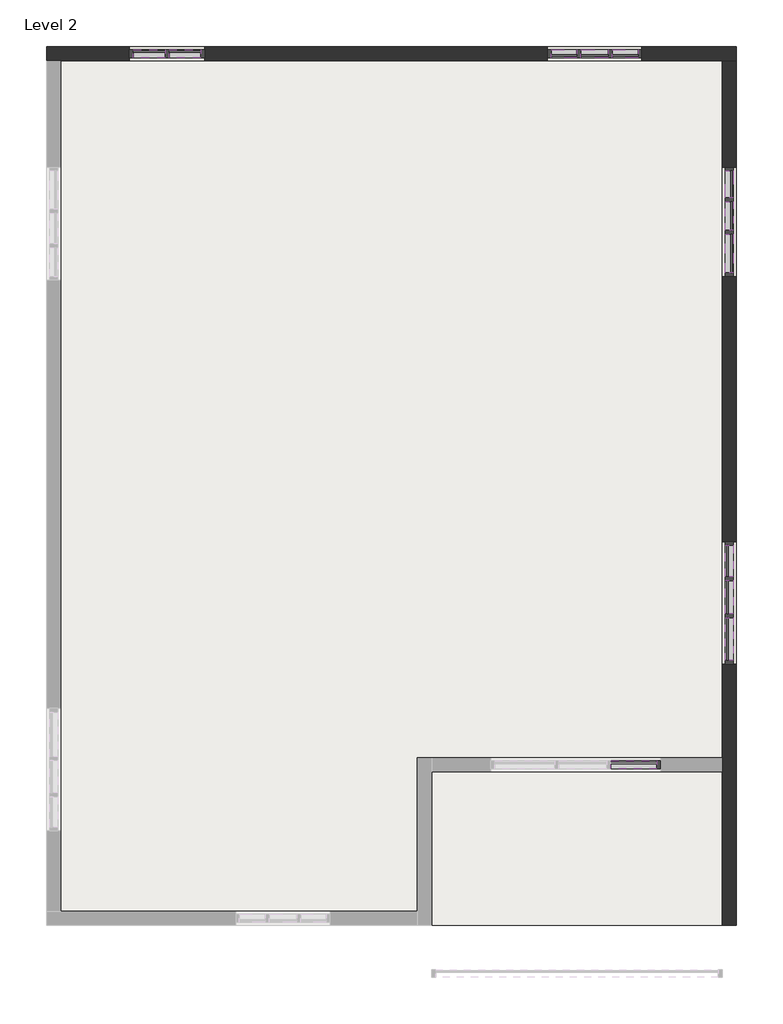
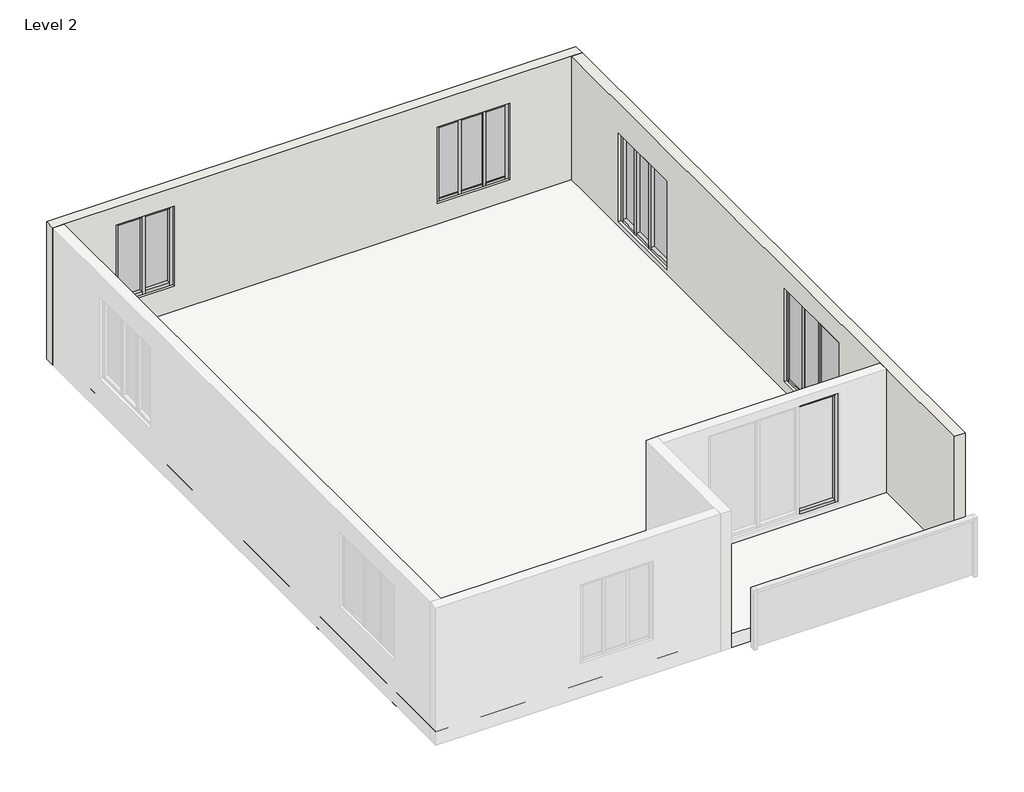
# One storey, part 2 of 2: 40 members, 11 plates, 2 walls, 1 roof.
"""IFC4 building model written with IfcOpenShell, lengths in millimetres."""

from ifc_helpers import new_model, si_unit, frame, origin, place, context, project, spatial, polyline, outline, extrude, faceted_brep, transform, mapped, element, save
from components import member_dc106669, member_0b7646a3, member_5f1d7e17, member_3f0e0172, member_3a0a7659, member_e878716d, member_b281fab0, member_45f9c1ec, member_8ea2817a, member_8eaddbd8, member_5535eeb3, member_69a911c1, member_1f3b6741, member_0bd10330, member_bc7dbe04, member_cf2a6f2c, member_fe0bf6b7, member_58f5e783, member_c04b3d4e, system_panel_glazed_4740d582, system_panel_glazed_d76279c0, system_panel_glazed_83f38206, system_panel_glazed_f7c25410, system_panel_glazed_1587745b, system_panel_glazed_2a40583e, system_panel_glazed_9aad7cd6, system_panel_glazed_e232d9b5, system_panel_glazed_0947b60d

model = new_model("IFC4")

# Units and contexts
model_context = context("Model", 3, world=origin())
ifc_project = project(units=[si_unit("LENGTHUNIT", "METRE", prefix="MILLI")], contexts=[model_context])

# Site, building, storey
site = spatial("IfcSite", under=ifc_project)
building = spatial("IfcBuilding", under=site)
storey = spatial("IfcBuildingStorey", under=building, Name="Level 2", Elevation=3048.0)

# Members
placement = place(None, origin())
member_shape = member_dc106669(model_context)
element("IfcMember", 1, ObjectType="Rectangular Mullion : 2.5\" x 5\" rectangular", at=placement, inside=storey, context=model_context, shape_type="MappedRepresentation", body=[
    mapped(member_shape, transform((-7605.3781629, -790.0678064, 5503.2729534), x_axis=(0.0, 0.0, 1.0), y_axis=(0.0, 1.0, 0.0), z_axis=(-1.0, 0.0, 0.0))),
])
element("IfcMember", 2, ObjectType="Rectangular Mullion : 2.5\" x 5\" rectangular", at=placement, inside=storey, context=model_context, shape_type="MappedRepresentation", body=[
    mapped(member_shape, transform((-8589.6281629, -790.0678064, 5503.2729534), x_axis=(0.0, 0.0, 1.0), y_axis=(0.0, 1.0, 0.0), z_axis=(-1.0, 0.0, 0.0))),
])
element("IfcMember", 3, ObjectType="Rectangular Mullion : 2.5\" x 5\" rectangular", at=placement, inside=storey, context=model_context, shape_type="MappedRepresentation", body=[
    mapped(member_shape, transform((-8176.8781629, -790.0678064, 3807.0200841), x_axis=(0.0, 0.0, -1.0), y_axis=(0.0, 1.0, 0.0), z_axis=(1.0, 0.0, 0.0))),
])
element("IfcMember", 4, ObjectType="Rectangular Mullion : 2.5\" x 5\" rectangular", at=placement, inside=storey, context=model_context, shape_type="MappedRepresentation", body=[
    mapped(member_shape, transform((-7192.6281629, -790.0678064, 3807.0200841), x_axis=(0.0, 0.0, -1.0), y_axis=(0.0, 1.0, 0.0), z_axis=(1.0, 0.0, 0.0))),
])
member_2_shape = member_0b7646a3(model_context)
element("IfcMember", 5, ObjectType="Rectangular Mullion : 2.5\" x 5\" rectangular", at=placement, inside=storey, context=model_context, shape_type="MappedRepresentation", body=[
    mapped(member_2_shape, transform((-14818.9781629, -790.0678064, 5692.341576), x_axis=(0.0, 0.0, 1.0), y_axis=(0.0, -1.0, 0.0), z_axis=(1.0, 0.0, 0.0))),
])
element("IfcMember", 6, ObjectType="Rectangular Mullion : 2.5\" x 5\" rectangular", at=placement, inside=storey, context=model_context, shape_type="MappedRepresentation", body=[
    mapped(member_2_shape, transform((-14241.1281629, -790.0678064, 5692.341576), x_axis=(0.0, 0.0, 1.0), y_axis=(0.0, -1.0, 0.0), z_axis=(1.0, 0.0, 0.0))),
])
element("IfcMember", 7, ObjectType="Rectangular Mullion : 2.5\" x 5\" rectangular", at=placement, inside=storey, context=model_context, shape_type="MappedRepresentation", body=[
    mapped(member_2_shape, transform((-14755.4781629, -790.0678064, 3913.1194519), x_axis=(0.0, 0.0, -1.0), y_axis=(0.0, -1.0, 0.0), z_axis=(-1.0, 0.0, 0.0))),
])
element("IfcMember", 8, ObjectType="Rectangular Mullion : 2.5\" x 5\" rectangular", at=placement, inside=storey, context=model_context, shape_type="MappedRepresentation", body=[
    mapped(member_2_shape, transform((-15333.3281629, -790.0678064, 3913.1194519), x_axis=(0.0, 0.0, -1.0), y_axis=(0.0, -1.0, 0.0), z_axis=(-1.0, 0.0, 0.0))),
])
member_3_shape = member_5f1d7e17(model_context)
element("IfcMember", 9, ObjectType="Rectangular Mullion : 2.5\" x 5\" rectangular", at=placement, inside=storey, context=model_context, shape_type="MappedRepresentation", body=[
    mapped(member_3_shape, transform((-5719.4281629, -9883.2678064, 5635.9695852), x_axis=(0.0, 0.0, 1.0), y_axis=(1.0, 0.0, 0.0), z_axis=(0.0, 1.0, 0.0))),
])
element("IfcMember", 10, ObjectType="Rectangular Mullion : 2.5\" x 5\" rectangular", at=placement, inside=storey, context=model_context, shape_type="MappedRepresentation", body=[
    mapped(member_3_shape, transform((-5719.4281629, -10575.4178064, 3572.3548103), x_axis=(0.0, 0.0, -1.0), y_axis=(1.0, 0.0, 0.0), z_axis=(0.0, -1.0, 0.0))),
])
member_4_shape = member_3f0e0172(model_context)
element("IfcMember", 11, ObjectType="Rectangular Mullion : 2.5\" x 5\" rectangular", at=placement, inside=storey, context=model_context, shape_type="MappedRepresentation", body=[
    mapped(member_4_shape, transform((-5719.4281629, -3704.7178064, 3463.7409857), x_axis=(0.0, 0.0, -1.0), y_axis=(-1.0, 0.0, 0.0), z_axis=(0.0, 1.0, 0.0))),
])
member_5_shape = member_3a0a7659(model_context)
element("IfcMember", 12, ObjectType="Rectangular Mullion : 2.5\" x 5\" rectangular", at=placement, inside=storey, context=model_context, shape_type="MappedRepresentation", body=[
    mapped(member_5_shape, transform((-7630.7781629, -12258.1678064, 3466.2078322), x_axis=(0.0, 0.0, -1.0), y_axis=(0.0, -1.0, 0.0), z_axis=(-1.0, 0.0, 0.0))),
])
element("IfcMember", 13, ObjectType="Rectangular Mullion : 2.5\" x 5\" rectangular", at=placement, inside=storey, context=model_context, shape_type="MappedRepresentation", body=[
    mapped(member_5_shape, transform((-6887.8281629, -12258.1678064, 5911.9599258), x_axis=(0.0, 0.0, 1.0), y_axis=(0.0, -1.0, 0.0), z_axis=(1.0, 0.0, 0.0))),
])
element("IfcMember", 14, ObjectType="Rectangular Mullion : 2.5\" x 5\" rectangular", at=placement, inside=storey, context=model_context, shape_type="MappedRepresentation", body=[
    mapped(member_4_shape, transform((-5719.4281629, -4320.6678064, 5428.2301601), x_axis=(0.0, 0.0, 1.0), y_axis=(-1.0, 0.0, 0.0), z_axis=(0.0, -1.0, 0.0))),
])
member_6_shape = member_e878716d(model_context)
element("IfcMember", 15, ObjectType="Rectangular Mullion : 2.5\" x 5\" rectangular", at=placement, inside=storey, context=model_context, shape_type="MappedRepresentation", body=[
    mapped(member_6_shape, transform((-6824.3281629, -12258.1678064, 3466.2078322), x_axis=(1.0, 0.0, 0.0), y_axis=(0.0, -1.0, 0.0), z_axis=(0.0, 0.0, -1.0))),
])
member_7_shape = member_b281fab0(model_context)
element("IfcMember", 16, ObjectType="Rectangular Mullion : 2.5\" x 5\" rectangular", at=placement, inside=storey, context=model_context, shape_type="MappedRepresentation", body=[
    mapped(member_7_shape, transform((-5719.4281629, -9286.3678064, 5635.9695852), x_axis=(0.0, 0.0, 1.0), y_axis=(1.0, 0.0, 0.0), z_axis=(0.0, 1.0, 0.0))),
])
member_8_shape = member_45f9c1ec(model_context)
element("IfcMember", 17, ObjectType="Rectangular Mullion : 2.5\" x 5\" rectangular", at=placement, inside=storey, context=model_context, shape_type="MappedRepresentation", body=[
    mapped(member_8_shape, transform((-5719.4281629, -8721.2178064, 5635.9695852), x_axis=(0.0, 0.0, 1.0), y_axis=(1.0, 0.0, 0.0), z_axis=(0.0, 1.0, 0.0))),
])
member_9_shape = member_8ea2817a(model_context)
element("IfcMember", 18, ObjectType="Rectangular Mullion : 2.5\" x 5\" rectangular", at=placement, inside=storey, context=model_context, shape_type="MappedRepresentation", body=[
    mapped(member_9_shape, transform((-5719.4281629, -9254.6178064, 3572.3548103), x_axis=(0.0, 1.0, 0.0), y_axis=(1.0, 0.0, 0.0), z_axis=(0.0, 0.0, -1.0))),
])
element("IfcMember", 19, ObjectType="Rectangular Mullion : 2.5\" x 5\" rectangular", at=placement, inside=storey, context=model_context, shape_type="MappedRepresentation", body=[
    mapped(member_9_shape, transform((-5719.4281629, -9851.5178064, 3572.3548103), x_axis=(0.0, 1.0, 0.0), y_axis=(1.0, 0.0, 0.0), z_axis=(0.0, 0.0, -1.0))),
])
element("IfcMember", 20, ObjectType="Rectangular Mullion : 2.5\" x 5\" rectangular", at=placement, inside=storey, context=model_context, shape_type="MappedRepresentation", body=[
    mapped(member_8_shape, transform((-5719.4281629, -9222.8678064, 3572.3548103), x_axis=(0.0, 0.0, -1.0), y_axis=(1.0, 0.0, 0.0), z_axis=(0.0, -1.0, 0.0))),
])
element("IfcMember", 21, ObjectType="Rectangular Mullion : 2.5\" x 5\" rectangular", at=placement, inside=storey, context=model_context, shape_type="MappedRepresentation", body=[
    mapped(member_7_shape, transform((-5719.4281629, -9819.7678064, 3572.3548103), x_axis=(0.0, 0.0, -1.0), y_axis=(1.0, 0.0, 0.0), z_axis=(0.0, -1.0, 0.0))),
])
member_10_shape = member_8eaddbd8(model_context)
element("IfcMember", 22, ObjectType="Rectangular Mullion : 2.5\" x 5\" rectangular", at=placement, inside=storey, context=model_context, shape_type="MappedRepresentation", body=[
    mapped(member_10_shape, transform((-5719.4281629, -8657.7178064, 3572.3548103), x_axis=(0.0, 1.0, 0.0), y_axis=(1.0, 0.0, 0.0), z_axis=(0.0, 0.0, -1.0))),
])
element("IfcMember", 23, ObjectType="Rectangular Mullion : 2.5\" x 5\" rectangular", at=placement, inside=storey, context=model_context, shape_type="MappedRepresentation", body=[
    mapped(member_10_shape, transform((-5719.4281629, -10638.9178064, 5635.9695852), x_axis=(0.0, -1.0, 0.0), y_axis=(1.0, 0.0, 0.0), z_axis=(0.0, 0.0, 1.0))),
])
member_11_shape = member_5535eeb3(model_context)
element("IfcMember", 24, ObjectType="Rectangular Mullion : 2.5\" x 5\" rectangular", at=placement, inside=storey, context=model_context, shape_type="MappedRepresentation", body=[
    mapped(member_11_shape, transform((-5719.4281629, -3177.6678064, 3463.7409857), x_axis=(0.0, 0.0, -1.0), y_axis=(-1.0, 0.0, 0.0), z_axis=(0.0, 1.0, 0.0))),
])
member_12_shape = member_69a911c1(model_context)
element("IfcMember", 25, ObjectType="Rectangular Mullion : 2.5\" x 5\" rectangular", at=placement, inside=storey, context=model_context, shape_type="MappedRepresentation", body=[
    mapped(member_12_shape, transform((-5719.4281629, -2682.3678064, 3463.7409857), x_axis=(0.0, 0.0, -1.0), y_axis=(-1.0, 0.0, 0.0), z_axis=(0.0, 1.0, 0.0))),
])
member_13_shape = member_1f3b6741(model_context)
element("IfcMember", 26, ObjectType="Rectangular Mullion : 2.5\" x 5\" rectangular", at=placement, inside=storey, context=model_context, shape_type="MappedRepresentation", body=[
    mapped(member_13_shape, transform((-5719.4281629, -3145.9178064, 3463.7409857), x_axis=(0.0, -1.0, 0.0), y_axis=(-1.0, 0.0, 0.0), z_axis=(0.0, 0.0, -1.0))),
])
element("IfcMember", 27, ObjectType="Rectangular Mullion : 2.5\" x 5\" rectangular", at=placement, inside=storey, context=model_context, shape_type="MappedRepresentation", body=[
    mapped(member_13_shape, transform((-5719.4281629, -3672.9678064, 3463.7409857), x_axis=(0.0, -1.0, 0.0), y_axis=(-1.0, 0.0, 0.0), z_axis=(0.0, 0.0, -1.0))),
])
element("IfcMember", 28, ObjectType="Rectangular Mullion : 2.5\" x 5\" rectangular", at=placement, inside=storey, context=model_context, shape_type="MappedRepresentation", body=[
    mapped(member_12_shape, transform((-5719.4281629, -3114.1678064, 5428.2301601), x_axis=(0.0, 0.0, 1.0), y_axis=(-1.0, 0.0, 0.0), z_axis=(0.0, -1.0, 0.0))),
])
element("IfcMember", 29, ObjectType="Rectangular Mullion : 2.5\" x 5\" rectangular", at=placement, inside=storey, context=model_context, shape_type="MappedRepresentation", body=[
    mapped(member_11_shape, transform((-5719.4281629, -3641.2178064, 5428.2301601), x_axis=(0.0, 0.0, 1.0), y_axis=(-1.0, 0.0, 0.0), z_axis=(0.0, -1.0, 0.0))),
])
member_14_shape = member_0bd10330(model_context)
element("IfcMember", 30, ObjectType="Rectangular Mullion : 2.5\" x 5\" rectangular", at=placement, inside=storey, context=model_context, shape_type="MappedRepresentation", body=[
    mapped(member_14_shape, transform((-5719.4281629, -2618.8678064, 5428.2301601), x_axis=(0.0, 1.0, 0.0), y_axis=(-1.0, 0.0, 0.0), z_axis=(0.0, 0.0, 1.0))),
])
element("IfcMember", 31, ObjectType="Rectangular Mullion : 2.5\" x 5\" rectangular", at=placement, inside=storey, context=model_context, shape_type="MappedRepresentation", body=[
    mapped(member_14_shape, transform((-5719.4281629, -4384.1678064, 3463.7409857), x_axis=(0.0, -1.0, 0.0), y_axis=(-1.0, 0.0, 0.0), z_axis=(0.0, 0.0, -1.0))),
])
member_15_shape = member_bc7dbe04(model_context)
element("IfcMember", 32, ObjectType="Rectangular Mullion : 2.5\" x 5\" rectangular", at=placement, inside=storey, context=model_context, shape_type="MappedRepresentation", body=[
    mapped(member_15_shape, transform((-7668.8781629, -790.0678064, 3807.0200841), x_axis=(0.0, 0.0, -1.0), y_axis=(0.0, 1.0, 0.0), z_axis=(1.0, 0.0, 0.0))),
])
member_16_shape = member_cf2a6f2c(model_context)
element("IfcMember", 33, ObjectType="Rectangular Mullion : 2.5\" x 5\" rectangular", at=placement, inside=storey, context=model_context, shape_type="MappedRepresentation", body=[
    mapped(member_16_shape, transform((-7637.1281629, -790.0678064, 3807.0200841), x_axis=(-1.0, 0.0, 0.0), y_axis=(0.0, 1.0, 0.0), z_axis=(0.0, 0.0, -1.0))),
])
element("IfcMember", 34, ObjectType="Rectangular Mullion : 2.5\" x 5\" rectangular", at=placement, inside=storey, context=model_context, shape_type="MappedRepresentation", body=[
    mapped(member_16_shape, transform((-8145.1281629, -790.0678064, 3807.0200841), x_axis=(-1.0, 0.0, 0.0), y_axis=(0.0, 1.0, 0.0), z_axis=(0.0, 0.0, -1.0))),
])
element("IfcMember", 35, ObjectType="Rectangular Mullion : 2.5\" x 5\" rectangular", at=placement, inside=storey, context=model_context, shape_type="MappedRepresentation", body=[
    mapped(member_15_shape, transform((-8113.3781629, -790.0678064, 5503.2729534), x_axis=(0.0, 0.0, 1.0), y_axis=(0.0, 1.0, 0.0), z_axis=(-1.0, 0.0, 0.0))),
])
member_17_shape = member_fe0bf6b7(model_context)
element("IfcMember", 36, ObjectType="Rectangular Mullion : 2.5\" x 5\" rectangular", at=placement, inside=storey, context=model_context, shape_type="MappedRepresentation", body=[
    mapped(member_17_shape, transform((-8653.1281629, -790.0678064, 3807.0200841), x_axis=(-1.0, 0.0, 0.0), y_axis=(0.0, 1.0, 0.0), z_axis=(0.0, 0.0, -1.0))),
])
element("IfcMember", 37, ObjectType="Rectangular Mullion : 2.5\" x 5\" rectangular", at=placement, inside=storey, context=model_context, shape_type="MappedRepresentation", body=[
    mapped(member_17_shape, transform((-7129.1281629, -790.0678064, 5503.2729534), x_axis=(1.0, 0.0, 0.0), y_axis=(0.0, 1.0, 0.0), z_axis=(0.0, 0.0, 1.0))),
])
member_18_shape = member_58f5e783(model_context)
element("IfcMember", 38, ObjectType="Rectangular Mullion : 2.5\" x 5\" rectangular", at=placement, inside=storey, context=model_context, shape_type="MappedRepresentation", body=[
    mapped(member_18_shape, transform((-14787.2281629, -790.0678064, 3913.1194519), x_axis=(1.0, 0.0, 0.0), y_axis=(0.0, -1.0, 0.0), z_axis=(0.0, 0.0, -1.0))),
])
member_19_shape = member_c04b3d4e(model_context)
element("IfcMember", 39, ObjectType="Rectangular Mullion : 2.5\" x 5\" rectangular", at=placement, inside=storey, context=model_context, shape_type="MappedRepresentation", body=[
    mapped(member_19_shape, transform((-15396.8281629, -790.0678064, 5692.341576), x_axis=(-1.0, 0.0, 0.0), y_axis=(0.0, -1.0, 0.0), z_axis=(0.0, 0.0, 1.0))),
])
element("IfcMember", 40, ObjectType="Rectangular Mullion : 2.5\" x 5\" rectangular", at=placement, inside=storey, context=model_context, shape_type="MappedRepresentation", body=[
    mapped(member_19_shape, transform((-14177.6281629, -790.0678064, 3913.1194519), x_axis=(1.0, 0.0, 0.0), y_axis=(0.0, -1.0, 0.0), z_axis=(0.0, 0.0, -1.0))),
])

# Plates
system_panel_glazed_shape = system_panel_glazed_4740d582(model_context)
element("IfcPlate", 41, ObjectType="System Panel : Glazed", at=placement, inside=storey, context=model_context, shape_type="MappedRepresentation", body=[
    mapped(system_panel_glazed_shape, transform((-5719.4281629, -10229.3428064, 3635.8548103), x_axis=(0.0, 1.0, 0.0), y_axis=(-1.0, 0.0, 0.0), z_axis=(0.0, 0.0, 1.0))),
])
system_panel_glazed_2_shape = system_panel_glazed_d76279c0(model_context)
element("IfcPlate", 42, ObjectType="System Panel : Glazed", at=placement, inside=storey, context=model_context, shape_type="MappedRepresentation", body=[
    mapped(system_panel_glazed_2_shape, transform((-5719.4281629, -9553.0678064, 3635.8548103), x_axis=(0.0, 1.0, 0.0), y_axis=(-1.0, 0.0, 0.0), z_axis=(0.0, 0.0, 1.0))),
])
system_panel_glazed_3_shape = system_panel_glazed_83f38206(model_context)
element("IfcPlate", 43, ObjectType="System Panel : Glazed", at=placement, inside=storey, context=model_context, shape_type="MappedRepresentation", body=[
    mapped(system_panel_glazed_3_shape, transform((-5719.4281629, -8972.0428064, 3635.8548103), x_axis=(0.0, 1.0, 0.0), y_axis=(-1.0, 0.0, 0.0), z_axis=(0.0, 0.0, 1.0))),
])
system_panel_glazed_4_shape = system_panel_glazed_f7c25410(model_context)
element("IfcPlate", 44, ObjectType="System Panel : Glazed", at=placement, inside=storey, context=model_context, shape_type="MappedRepresentation", body=[
    mapped(system_panel_glazed_4_shape, transform((-5719.4281629, -2898.2678064, 3527.2409857), x_axis=(0.0, -1.0, 0.0), y_axis=(1.0, 0.0, 0.0), z_axis=(0.0, 0.0, 1.0))),
])
system_panel_glazed_5_shape = system_panel_glazed_1587745b(model_context)
element("IfcPlate", 45, ObjectType="System Panel : Glazed", at=placement, inside=storey, context=model_context, shape_type="MappedRepresentation", body=[
    mapped(system_panel_glazed_5_shape, transform((-5719.4281629, -4012.6928064, 3527.2409857), x_axis=(0.0, -1.0, 0.0), y_axis=(1.0, 0.0, 0.0), z_axis=(0.0, 0.0, 1.0))),
])
system_panel_glazed_6_shape = system_panel_glazed_2a40583e(model_context)
element("IfcPlate", 46, ObjectType="System Panel : Glazed", at=placement, inside=storey, context=model_context, shape_type="MappedRepresentation", body=[
    mapped(system_panel_glazed_6_shape, transform((-5719.4281629, -3409.4428064, 3527.2409857), x_axis=(0.0, -1.0, 0.0), y_axis=(1.0, 0.0, 0.0), z_axis=(0.0, 0.0, 1.0))),
])
system_panel_glazed_7_shape = system_panel_glazed_9aad7cd6(model_context)
element("IfcPlate", 47, ObjectType="System Panel : Glazed", at=placement, inside=storey, context=model_context, shape_type="MappedRepresentation", body=[
    mapped(system_panel_glazed_7_shape, transform((-7399.0031629, -790.0678064, 3870.5200841), x_axis=(-1.0, 0.0, 0.0), y_axis=(0.0, -1.0, 0.0), z_axis=(0.0, 0.0, 1.0))),
])
element("IfcPlate", 48, ObjectType="System Panel : Glazed", at=placement, inside=storey, context=model_context, shape_type="MappedRepresentation", body=[
    mapped(system_panel_glazed_7_shape, transform((-8383.2531629, -790.0678064, 3870.5200841), x_axis=(-1.0, 0.0, 0.0), y_axis=(0.0, -1.0, 0.0), z_axis=(0.0, 0.0, 1.0))),
])
system_panel_glazed_8_shape = system_panel_glazed_e232d9b5(model_context)
element("IfcPlate", 49, ObjectType="System Panel : Glazed", at=placement, inside=storey, context=model_context, shape_type="MappedRepresentation", body=[
    mapped(system_panel_glazed_8_shape, transform((-7891.1281629, -790.0678064, 3870.5200841), x_axis=(-1.0, 0.0, 0.0), y_axis=(0.0, -1.0, 0.0), z_axis=(0.0, 0.0, 1.0))),
])
system_panel_glazed_9_shape = system_panel_glazed_0947b60d(model_context)
element("IfcPlate", 50, ObjectType="System Panel : Glazed", at=placement, inside=storey, context=model_context, shape_type="MappedRepresentation", body=[
    mapped(system_panel_glazed_9_shape, transform((-15076.1531629, -790.0678064, 3976.6194519), x_axis=(1.0, 0.0, 0.0), y_axis=(0.0, 1.0, 0.0), z_axis=(0.0, 0.0, 1.0))),
])
element("IfcPlate", 51, ObjectType="System Panel : Glazed", at=placement, inside=storey, context=model_context, shape_type="MappedRepresentation", body=[
    mapped(system_panel_glazed_9_shape, transform((-14498.3031629, -790.0678064, 3976.6194519), x_axis=(1.0, 0.0, 0.0), y_axis=(0.0, 1.0, 0.0), z_axis=(0.0, 0.0, 1.0))),
])

# Roof
element("IfcRoof", 52, ObjectType="Generic - 12\"", at=placement, inside=storey, context=model_context, shape_type="SweptSolid", body=[
    extrude(outline(polyline([(-16730.3281629, -675.7678064), (-5605.1281629, -675.7678064), (-5605.1281629, -14848.9678064), (-16730.3281629, -14848.9678064), (-16730.3281629, -675.7678064)])), frame((0.0, 0.0, 3048.0), z_axis=(0.0, 0.0, 1.0), x_axis=(1.0, 0.0, 0.0)), (0.0, 0.0, 1.0), 304.8),
])

# Walls
element("IfcWall", 53, ObjectType="9\"", at=placement, inside=storey, context=model_context, shape_type="Brep", body=[
    faceted_brep([(-16730.3281629, -904.3678064, 3048.0), (-16501.7281629, -904.3678064, 3048.0), (-5833.7281629, -904.3678064, 3048.0), (-5605.1281629, -904.3678064, 3048.0), (-5605.1281629, -904.3678064, 6096.0), (-5833.7281629, -904.3678064, 6096.0), (-16501.7281629, -904.3678064, 6096.0), (-16730.3281629, -904.3678064, 6096.0), (-7129.1281629, -904.3678064, 5503.2729534), (-7129.1281629, -904.3678064, 3807.0200841), (-8653.1281629, -904.3678064, 3807.0200841), (-8653.1281629, -904.3678064, 5503.2729534), (-15396.8281629, -904.3678064, 3913.1194519), (-15396.8281629, -904.3678064, 5692.341576), (-14177.6281629, -904.3678064, 5692.341576), (-14177.6281629, -904.3678064, 3913.1194519), (-5605.1281629, -675.7678064, 3048.0), (-16730.3281629, -675.7678064, 3048.0), (-16730.3281629, -675.7678064, 6096.0), (-5605.1281629, -675.7678064, 6096.0), (-7129.1281629, -675.7678064, 3807.0200841), (-7129.1281629, -675.7678064, 5503.2729534), (-8653.1281629, -675.7678064, 5503.2729534), (-8653.1281629, -675.7678064, 3807.0200841), (-15396.8281629, -675.7678064, 5692.341576), (-15396.8281629, -675.7678064, 3913.1194519), (-14177.6281629, -675.7678064, 3913.1194519), (-14177.6281629, -675.7678064, 5692.341576)], [[[0, 1, 2, 3, 4, 5, 6, 7], [8, 9, 10, 11], [12, 13, 14, 15]], [[16, 17, 18, 19], [20, 21, 22, 23], [24, 25, 26, 27]], [[3, 2, 1, 0, 17, 16]], [[7, 6, 5, 4, 19, 18]], [[0, 7, 18, 17]], [[4, 3, 16, 19]], [[8, 21, 20, 9]], [[21, 8, 11, 22]], [[22, 11, 10, 23]], [[9, 20, 23, 10]], [[12, 25, 24, 13]], [[13, 24, 27, 14]], [[14, 27, 26, 15]], [[25, 12, 15, 26]]]),
])
element("IfcWall", 54, ObjectType="9\"", at=placement, inside=storey, context=model_context, shape_type="Brep", body=[
    faceted_brep([(-5833.7281629, -904.3678064, 3048.0), (-5833.7281629, -12143.8678064, 3048.0), (-5833.7281629, -12372.4678064, 3048.0), (-5833.7281629, -14848.9678064, 3048.0), (-5833.7281629, -14848.9678064, 6096.0), (-5833.7281629, -12372.4678064, 6096.0), (-5833.7281629, -12143.8678064, 6096.0), (-5833.7281629, -904.3678064, 6096.0), (-5833.7281629, -10638.9178064, 5635.9695852), (-5833.7281629, -10638.9178064, 3572.3548103), (-5833.7281629, -8657.7178064, 3572.3548103), (-5833.7281629, -8657.7178064, 5635.9695852), (-5833.7281629, -2618.8678064, 3463.7409857), (-5833.7281629, -2618.8678064, 5428.2301601), (-5833.7281629, -4384.1678064, 5428.2301601), (-5833.7281629, -4384.1678064, 3463.7409857), (-5605.1281629, -14848.9678064, 3048.0), (-5605.1281629, -904.3678064, 3048.0), (-5605.1281629, -904.3678064, 6096.0), (-5605.1281629, -14848.9678064, 6096.0), (-5605.1281629, -10638.9178064, 3572.3548103), (-5605.1281629, -10638.9178064, 5635.9695852), (-5605.1281629, -8657.7178064, 5635.9695852), (-5605.1281629, -8657.7178064, 3572.3548103), (-5605.1281629, -2618.8678064, 5428.2301601), (-5605.1281629, -2618.8678064, 3463.7409857), (-5605.1281629, -4384.1678064, 3463.7409857), (-5605.1281629, -4384.1678064, 5428.2301601)], [[[0, 1, 2, 3, 4, 5, 6, 7], [8, 9, 10, 11], [12, 13, 14, 15]], [[16, 17, 18, 19], [20, 21, 22, 23], [24, 25, 26, 27]], [[3, 2, 1, 0, 17, 16]], [[4, 3, 16, 19]], [[7, 6, 5, 4, 19, 18]], [[0, 7, 18, 17]], [[8, 21, 20, 9]], [[21, 8, 11, 22]], [[22, 11, 10, 23]], [[9, 20, 23, 10]], [[12, 25, 24, 13]], [[13, 24, 27, 14]], [[14, 27, 26, 15]], [[25, 12, 15, 26]]]),
])

save(model, "model.ifc")

# Revit data of these elements
# Type "Rectangular Mullion : 2.5\" x 5\" rectangular"
#   built-in parameter 1007304 = 0.416667 (stored number, unit not read)
#   built-in parameter 1007301 = 0.104167 (stored number, unit not read)
#   built-in parameter 1007300 = 0.104167 (stored number, unit not read)
# Type "System Panel : Glazed"
#   Construction Type Id = "GSP4R"
#   Analytic Construction = "1/8 in Pilkington single glazing"
#   Visual Light Transmittance = 0.9
#   Solar Heat Gain Coefficient = 0.86
#   Heat Transfer Coefficient (U) = 1.18115 BTU/(h·ft²·°F)
#   Define Thermal Properties by = 1
# Type "Generic - 12\""
#   Assembly Code = "B1020"
#   Layers, outside or top first: 1' - 0" no material (function 1)
# Type "9\""
#   Assembly Code = "B2010"
#   Layers, outside or top first: 0' - 9" no material (function 1)
# Elements 1, 2, 3, 4, 5, 6, 7, 8, 9, 10, 11, 12, 13, 14, 15, 16, 17, 18, 19, 20, 21, 22, 23, 24, 25, 26, 27, 28, 29, 30, 31, 32, 33, 34, 35, 36, 37, 38, 39, 40 (IfcMember, "Rectangular Mullion : 2.5\" x 5\" rectangular")
#   Phase Created = New Construction
#   Materials on its faces: "Aluminum"
# Elements 41, 42, 43, 44, 45, 46, 47, 48, 49, 50, 51 (IfcPlate, "System Panel : Glazed")
#   Phase Created = New Construction
#   Materials on its faces: "Glass"
# Element 52 (IfcRoof, "Generic - 12\"")
#   built-in parameter 1001705 = 11 (stored number, unit not read)
#   built-in parameter 1001710 = 33615
#   Phase Created = New Construction
#   Materials on its faces: "Default Roof"
# Elements 53, 54 (IfcWall, "9\"")
#   Top Offset = 0' - 0"
#   Base Offset = 0' - 0"
#   Unconnected Height = 10' - 0"
#   wall height = 10' - 0"
#   Phase Created = New Construction
#   Base Constraint = Level 2
#   Materials on its faces: "Default Wall"
# Materials
#   "Aluminum": class "Metal", colour RGB 247 247 247, transparency 0, Description = "Aluminum 6061", Cost = 0
#   "Glass": class "Glass", colour RGB 0 128 192, transparency 0.75, Description = "Soda Lime Glass", Cost = 0
#   "Default Roof": colour RGB 88 101 114, transparency 0, Cost = 0
#   "Default Wall": colour RGB 128 128 128, transparency 0, Cost = 0
